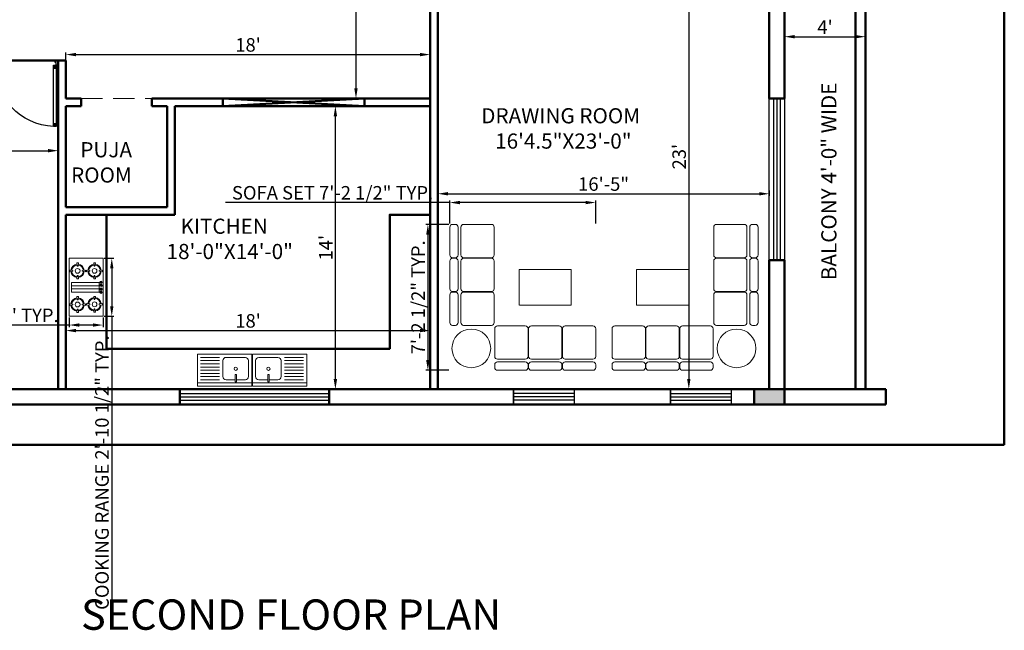
# Model space of a CAD drawing. Units: millimetres. Extents: x 1706 to 5913, y 156 to 1716.
# Tile 3 of 26: x 2060 to 2643, y 211 to 573. Entities that reach past the tile are written whole.
import ezdxf

# ---------------------------------------------------------------- set-up
doc = ezdxf.new("R2010")
doc.units = ezdxf.units.MM
doc.linetypes.add('DASHED', pattern=[19.05, 12.7, -6.35])
for name, color, linetype, lineweight in [('A-ANNO-DIMS', 2, 'Continuous', 18), ('A-ANNO-TEXT', 7, 'Continuous', 18), ('A-AREA-IDEN', 3, 'Continuous', 18), ('A-COLS', 20, 'Continuous', 50), ('A-DOOR', 4, 'Continuous', 25), ('A-FLOR-OVHD', 9, 'DASHED', 18), ('A-FURN', 8, 'Continuous', 18), ('A-GLAZ', 150, 'Continuous', 25), ('A-WALL', 7, 'Continuous', 50)]:
    doc.layers.add(name, color=color, linetype=linetype, lineweight=lineweight)
doc.styles.get("Standard").update_dxf_attribs({"font": 'arial.ttf'})
doc.dimstyles.new('ISO-25', dxfattribs={"dimtxt": 8, "dimasz": 6, "dimexe": 1.25, "dimexo": 0.625, "dimtad": 1, "dimdec": 0, "dimlunit": 3, "dimtxsty": 'Standard', "dimcen": 2.5, "dimadec": 0, "dimazin": 0, "dimtfac": 1, "dimtdec": 0, "dimtmove": 0, "dimatfit": 3, "dimfxl": 1, "dimarcsym": 0})

# ---------------------------------------------------------------- blocks, each defined once
blk = doc.blocks.new('Puerta 01')
for p, q in [((-0.775, -0.026), (-0.737, -0.058)), ((-0.775, -0.058), (-0.737, -0.026)), ((-0.737, -0.058), (-0.737, -0.026)), ((-0.028, -0.058), (-0.066, -0.026)), ((-0.028, -0.026), (-0.066, -0.058)), ((-0.066, -0.058), (-0.066, -0.026))]:
    blk.add_line(p, q)
for points in [[(-0.028, 0), (-0.028, -0.026), (0.004, -0.026), (0.004, -0.036), (0.028, -0.036), (0.028, 0)], [(-0.028, -0.026), (-0.775, -0.026), (-0.775, -0.058), (-0.028, -0.058)], [(0.004, -0.774), (0.004, -0.764), (0.028, -0.764), (0.028, -0.8), (-0.028, -0.8), (-0.028, -0.774)]]:
    blk.add_lwpolyline(points, close=True)
blk.add_arc((-0.028, -0.026), 0.747, 182.4545, 270)
blk = doc.blocks.new('A$C57CF26DA')
for p, q in [((0, 0), (0, 420)), ((720, 420), (0, 420)), ((167, 413), (147, 413)), ((147, 413), (152, 373)), ((152, 373), (162, 373)), ((162, 373), (167, 413)), ((300, 391), (300, 49)), ((300, 391), (420, 391)), ((340, 391), (340, 49)), ((380, 391), (380, 49)), ((420, 391), (420, 49)), ((584, 413), (564, 413)), ((564, 413), (569, 373)), ((569, 373), (579, 373)), ((579, 373), (584, 413)), ((720, 0), (720, 420)), ((99, 320), (59, 325)), ((59, 325), (59, 305)), ((59, 305), (99, 310)), ((99, 310), (99, 320)), ((152, 257), (147, 217)), ((162, 257), (152, 257)), ((167, 217), (162, 257)), ((255, 325), (215, 320)), ((215, 320), (215, 310)), ((215, 310), (255, 305)), ((255, 305), (255, 325)), ((516, 320), (476, 325)), ((476, 325), (476, 305)), ((476, 305), (516, 310)), ((516, 310), (516, 320)), ((569, 257), (564, 217)), ((579, 257), (569, 257)), ((584, 217), (579, 257)), ((672, 325), (632, 320)), ((632, 320), (632, 310)), ((632, 310), (672, 305)), ((672, 305), (672, 325)), ((147, 217), (167, 217)), ((167, 203), (147, 203)), ((147, 203), (152, 163)), ((152, 163), (162, 163)), ((162, 163), (167, 203)), ((581, 203), (561, 203)), ((561, 203), (566, 163)), ((564, 217), (584, 217)), ((566, 163), (576, 163)), ((576, 163), (581, 203)), ((99, 110), (59, 115)), ((59, 115), (59, 95)), ((59, 95), (99, 100)), ((99, 100), (99, 110)), ((152, 47), (147, 7)), ((147, 7), (167, 7)), ((162, 47), (152, 47)), ((167, 7), (162, 47)), ((255, 115), (215, 110)), ((215, 110), (215, 100)), ((215, 100), (255, 95)), ((255, 95), (255, 115)), ((302, 39), (295, 39)), ((295, 39), (295, 11)), ((295, 11), (302, 11)), ((420, 49), (300, 49)), ((302, 11), (302, 39)), ((341, 39), (334, 39)), ((334, 39), (334, 11)), ((334, 11), (341, 11)), ((341, 11), (341, 39)), ((380, 11), (380, 39)), ((380, 39), (386, 39)), ((386, 11), (380, 11)), ((386, 39), (386, 11)), ((419, 11), (419, 39)), ((419, 39), (426, 39)), ((426, 11), (419, 11)), ((426, 39), (426, 11)), ((513, 110), (473, 115)), ((473, 115), (473, 95)), ((473, 95), (513, 100)), ((513, 100), (513, 110)), ((566, 47), (561, 7)), ((561, 7), (581, 7)), ((576, 47), (566, 47)), ((581, 7), (576, 47)), ((669, 115), (629, 110)), ((629, 110), (629, 100)), ((629, 100), (669, 95)), ((669, 95), (669, 115)), ((720, 0), (0, 0))]:
    blk.add_line(p, q)
for centre in [(157, 315), (574, 315), (157, 105), (571, 105)]:
    blk.add_circle(centre, 30)
for centre, radius, start, end in [((157, 315), 83, 95.5849, 174.4151), ((157, 315), 73, 95.3738, 174.6262), ((157, 315), 73, 5.3738, 84.6262), ((157, 315), 83, 5.5849, 84.4151), ((574, 315), 83, 95.5849, 174.4151), ((574, 315), 73, 95.3738, 174.6262), ((574, 315), 73, 5.3738, 84.6262), ((574, 315), 83, 5.5849, 84.4151), ((157, 315), 83, 185.5849, 264.4151), ((157, 315), 73, 185.3738, 264.6262), ((157, 315), 73, 275.3738, 354.6262), ((157, 315), 83, 275.5849, 354.4151), ((574, 315), 83, 185.5849, 264.4151), ((574, 315), 73, 185.3738, 264.6262), ((574, 315), 73, 275.3738, 354.6262), ((574, 315), 83, 275.5849, 354.4151), ((157, 105), 83, 95.5849, 174.4151), ((157, 105), 73, 95.3738, 174.6262), ((157, 105), 73, 5.3738, 84.6262), ((157, 105), 83, 5.5849, 84.4151), ((571, 105), 83, 95.5849, 174.4151), ((571, 105), 73, 95.3738, 174.6262), ((571, 105), 73, 5.3738, 84.6262), ((571, 105), 83, 5.5849, 84.4151), ((157, 105), 83, 185.5849, 264.4151), ((157, 105), 73, 185.3738, 264.6262), ((157, 105), 73, 275.3738, 354.6262), ((157, 105), 83, 275.5849, 354.4151), ((298, 25), 13.7, 104.4775, 255.5225), ((298, 25), 13.7, 284.4775, 75.5225), ((337, 25), 13.7, 104.4775, 255.5225), ((337, 25), 13.7, 284.4775, 75.5225), ((383, 25), 13.7, 104.4775, 255.5225), ((383, 25), 13.7, 284.4775, 75.5225), ((422, 25), 13.7, 104.4775, 255.5225), ((422, 25), 13.7, 284.4775, 75.5225), ((571, 105), 83, 185.5849, 264.4151), ((571, 105), 73, 185.3738, 264.6262), ((571, 105), 73, 275.3738, 354.6262), ((571, 105), 83, 275.5849, 354.4151)]:
    blk.add_arc(centre, radius, start, end)
blk = doc.blocks.new('A$C3404121D')
for p, q in [((0, 0), (0, 500)), ((0, 500), (850, 500)), ((850, 500), (850, 0)), ((0, 450), (850, 450)), ((50, 100), (50, 350)), ((100, 400), (240, 400)), ((240, 431), (240, 425)), ((260, 431), (240, 431)), ((240, 425), (240, 315)), ((240, 315), (260, 315)), ((260, 431), (260, 315)), ((260, 400), (400, 400)), ((450, 100), (450, 350)), ((502, 400), (801, 400)), ((502, 350), (801, 350)), ((502, 300), (801, 300)), ((502, 250), (801, 250)), ((502, 200), (801, 200)), ((850, 0), (0, 0)), ((400, 50), (100, 50)), ((502, 150), (801, 150)), ((502, 100), (801, 100)), ((801, 50), (502, 50))]:
    blk.add_line(p, q)
blk.add_circle((250, 228), 25)
for centre, start, end in [((100, 350), 90, 180), ((400, 350), 0, 90), ((100, 100), 180, 270), ((400, 100), 270, 0)]:
    blk.add_arc(centre, 50, start, end)
blk = doc.blocks.new('A$C753D6792')
at = {"linetype": 'ByBlock'}
for p, q in [((0, 2530), (0, 2580)), ((50, 2630), (550, 2630)), ((600, 2580), (600, 2530)), ((610, 2530), (610, 2580)), ((660, 2630), (1160, 2630)), ((1210, 2580), (1210, 2530)), ((1220, 2530), (1220, 2580)), ((1270, 2630), (1770, 2630)), ((1820, 2580), (1820, 2530)), ((0, 1880), (0, 2380)), ((550, 2480), (50, 2480)), ((550, 2430), (50, 2430)), ((600, 2380), (600, 1880)), ((610, 1880), (610, 2380)), ((1160, 2480), (660, 2480)), ((1160, 2430), (660, 2430)), ((1210, 2380), (1210, 1880)), ((1220, 1880), (1220, 2380)), ((1770, 2480), (1270, 2480)), ((1770, 2430), (1270, 2430)), ((1820, 1880), (1820, 2380)), ((50, 1830), (427, 1830)), ((387, 1830), (550, 1830)), ((660, 1830), (1037, 1830)), ((997, 1830), (1160, 1830)), ((1270, 1830), (1647, 1830)), ((1607, 1830), (1770, 1830)), ((1880, 1820), (2380, 1820)), ((2530, 1820), (2580, 1820)), ((1830, 1770), (1830, 1393)), ((2430, 1270), (2430, 1770)), ((2480, 1270), (2480, 1770)), ((2630, 1770), (2630, 1270)), ((442, 815), (442, 1455)), ((442, 1455), (1372, 1455)), ((1382, 1455), (1382, 815)), ((1830, 1433), (1830, 1270)), ((1830, 1160), (1830, 783)), ((2380, 1220), (1880, 1220)), ((1880, 1210), (2380, 1210)), ((2430, 660), (2430, 1160)), ((2480, 660), (2480, 1160)), ((2580, 1220), (2530, 1220)), ((2530, 1210), (2580, 1210)), ((2630, 1160), (2630, 660)), ((1382, 815), (442, 815)), ((1830, 823), (1830, 660)), ((1830, 550), (1830, 173)), ((2380, 610), (1880, 610)), ((1880, 600), (2380, 600)), ((2430, 50), (2430, 550)), ((2480, 50), (2480, 550)), ((2580, 610), (2530, 610)), ((2530, 600), (2580, 600)), ((2630, 550), (2630, 50)), ((1830, 213), (1830, 50)), ((2380, 0), (1880, 0)), ((2580, 0), (2530, 0))]:
    blk.add_line(p, q, dxfattribs=at)
blk.add_circle((2242, 2235), 349, dxfattribs=at)
for centre, start, end in [((50, 2580), 90, 180), ((50, 2530), 180, 270), ((550, 2580), 0, 90), ((550, 2580), 0, 90), ((550, 2530), 270, 0), ((550, 2530), 270, 0), ((660, 2580), 90, 180), ((660, 2530), 180, 270), ((1160, 2580), 0, 90), ((1160, 2580), 0, 90), ((1160, 2530), 270, 0), ((1160, 2530), 270, 0), ((1270, 2580), 90, 180), ((1270, 2530), 180, 270), ((1770, 2580), 0, 90), ((1770, 2580), 0, 90), ((1770, 2530), 270, 0), ((1770, 2530), 270, 0), ((50, 2380), 90, 180), ((550, 2380), 0, 90), ((550, 2380), 0, 90), ((660, 2380), 90, 180), ((1160, 2380), 0, 90), ((1160, 2380), 0, 90), ((1270, 2380), 90, 180), ((1770, 2380), 0, 90), ((1770, 2380), 0, 90), ((50, 1880), 180, 270), ((550, 1880), 270, 0), ((660, 1880), 180, 270), ((1160, 1880), 270, 0), ((1270, 1880), 180, 270), ((1770, 1880), 270, 0), ((1880, 1770), 90, 180), ((2380, 1770), 0, 90), ((2530, 1770), 90, 180), ((2580, 1770), 0, 90), ((1880, 1270), 180, 270), ((2380, 1270), 270, 0), ((2380, 1270), 270, 0), ((2530, 1270), 180, 270), ((2530, 1270), 180, 270), ((2580, 1270), 270, 0), ((2580, 1270), 270, 0), ((1880, 1160), 90, 180), ((2380, 1160), 0, 90), ((2530, 1160), 90, 180), ((2580, 1160), 0, 90), ((1880, 660), 180, 270), ((1880, 550), 90, 180), ((2380, 660), 270, 0), ((2380, 660), 270, 0), ((2380, 550), 0, 90), ((2530, 660), 180, 270), ((2530, 660), 180, 270), ((2530, 550), 90, 180), ((2580, 660), 270, 0), ((2580, 660), 270, 0), ((2580, 550), 0, 90), ((1880, 50), 180, 270), ((2380, 50), 270, 0), ((2380, 50), 270, 0), ((2530, 50), 180, 270), ((2530, 50), 180, 270), ((2580, 50), 270, 0), ((2580, 50), 270, 0)]:
    blk.add_arc(centre, 50, start, end, dxfattribs=at)
blk = doc.blocks.new('*D119')
at = {"layer": 'A-ANNO-DIMS', "color": 0, "lineweight": -2, "transparency": 16777216}
for p, q in [((1801.94, 495.25), (1801.94, 496.83)), ((2082.44, 495.25), (2082.44, 496.83)), ((1807.94, 495.58), (2076.44, 495.58))]:
    blk.add_line(p, q, dxfattribs=at)
at = {"layer": 'A-ANNO-DIMS', "color": 0, "transparency": 16777216}
for points in [[(1807.94, 496.58), (1807.94, 494.58), (1801.94, 495.58)], [(2076.44, 496.58), (2076.44, 494.58), (2082.44, 495.58)]]:
    blk.add_solid(points, dxfattribs=at)
at = {"layer": 'Defpoints', "color": 0, "transparency": 16777216}
for p in [(1801.94, 494.63), (2082.44, 495.58), (2082.44, 494.63)]:
    blk.add_point(p, dxfattribs=at)
at = {"layer": 'A-ANNO-DIMS', "color": 0, "transparency": 16777216, "insert": (1942.19, 500.29), "char_height": 8, "attachment_point": 5}
blk.add_mtext('23\'-5"', dxfattribs=at)
blk = doc.blocks.new('*D136')
at = {"layer": 'A-ANNO-DIMS', "color": 0, "lineweight": -2, "transparency": 16777216}
for p, q in [((2256.32, 684.04), (2260.17, 684.04)), ((2258.92, 678.04), (2258.92, 532.54)), ((2256.32, 526.54), (2260.17, 526.54))]:
    blk.add_line(p, q, dxfattribs=at)
at = {"layer": 'A-ANNO-DIMS', "color": 0, "transparency": 16777216}
for points in [[(2257.92, 678.04), (2259.92, 678.04), (2258.92, 684.04)], [(2257.92, 532.54), (2259.92, 532.54), (2258.92, 526.54)]]:
    blk.add_solid(points, dxfattribs=at)
at = {"layer": 'Defpoints', "color": 0, "transparency": 16777216}
for p in [(2255.69, 684.04), (2255.69, 526.54), (2258.92, 526.54)]:
    blk.add_point(p, dxfattribs=at)
at = {"layer": 'A-ANNO-DIMS', "color": 0, "transparency": 16777216, "insert": (2254.2, 605.29), "char_height": 8, "attachment_point": 5, "rotation": 90}
blk.add_mtext('13\'-2"', dxfattribs=at)
blk = doc.blocks.new('*D137')
at = {"layer": 'A-ANNO-DIMS', "color": 0, "lineweight": -2, "transparency": 16777216}
for p, q in [((2086.94, 540.29), (2086.94, 553.85)), ((2092.94, 552.6), (2296.94, 552.6)), ((2302.94, 540.29), (2302.94, 553.85))]:
    blk.add_line(p, q, dxfattribs=at)
at = {"layer": 'A-ANNO-DIMS', "color": 0, "transparency": 16777216}
for points in [[(2092.94, 553.6), (2092.94, 551.6), (2086.94, 552.6)], [(2296.94, 553.6), (2296.94, 551.6), (2302.94, 552.6)]]:
    blk.add_solid(points, dxfattribs=at)
at = {"layer": 'Defpoints', "color": 0, "transparency": 16777216}
for p in [(2302.94, 552.6), (2086.94, 539.66), (2302.94, 539.66)]:
    blk.add_point(p, dxfattribs=at)
at = {"layer": 'A-ANNO-DIMS', "color": 0, "transparency": 16777216, "insert": (2194.94, 557.31), "char_height": 8, "attachment_point": 5}
blk.add_mtext("18'", dxfattribs=at)
blk = doc.blocks.new('*D138')
at = {"layer": 'A-ANNO-DIMS', "color": 0, "lineweight": -2, "transparency": 16777216}
for p, q in [((2247.7, 522.04), (2245.46, 522.04)), ((2246.71, 360.04), (2246.71, 516.04)), ((2247.7, 354.04), (2245.46, 354.04))]:
    blk.add_line(p, q, dxfattribs=at)
at = {"layer": 'A-ANNO-DIMS', "color": 0, "transparency": 16777216}
for points in [[(2245.71, 516.04), (2247.71, 516.04), (2246.71, 522.04)], [(2245.71, 360.04), (2247.71, 360.04), (2246.71, 354.04)]]:
    blk.add_solid(points, dxfattribs=at)
at = {"layer": 'Defpoints', "color": 0, "transparency": 16777216}
for p in [(2246.71, 522.04), (2248.33, 522.04), (2248.33, 354.04)]:
    blk.add_point(p, dxfattribs=at)
at = {"layer": 'A-ANNO-DIMS', "color": 0, "transparency": 16777216, "insert": (2242.07, 438.04), "char_height": 8, "attachment_point": 5, "rotation": 90}
blk.add_mtext("14'", dxfattribs=at)
blk = doc.blocks.new('*D139')
at = {"layer": 'A-ANNO-DIMS', "color": 0, "lineweight": -2, "transparency": 16777216}
for p, q in [((2086.94, 381.5), (2086.94, 390.09)), ((2092.94, 388.84), (2296.94, 388.84)), ((2302.94, 381.5), (2302.94, 390.09))]:
    blk.add_line(p, q, dxfattribs=at)
at = {"layer": 'A-ANNO-DIMS', "color": 0, "transparency": 16777216}
for points in [[(2092.94, 389.84), (2092.94, 387.84), (2086.94, 388.84)], [(2296.94, 389.84), (2296.94, 387.84), (2302.94, 388.84)]]:
    blk.add_solid(points, dxfattribs=at)
at = {"layer": 'Defpoints', "color": 0, "transparency": 16777216}
for p in [(2302.94, 388.84), (2086.94, 380.87), (2302.94, 380.87)]:
    blk.add_point(p, dxfattribs=at)
at = {"layer": 'A-ANNO-DIMS', "color": 0, "transparency": 16777216, "insert": (2194.94, 393.55), "char_height": 8, "attachment_point": 5}
blk.add_mtext("18'", dxfattribs=at)
blk = doc.blocks.new('*D140')
at = {"layer": 'A-ANNO-DIMS', "color": 0, "lineweight": -2, "transparency": 16777216}
for p, q in [((2452.75, 630.04), (2457.47, 630.04)), ((2456.22, 624.04), (2456.22, 360.04)), ((2452.75, 354.04), (2457.47, 354.04))]:
    blk.add_line(p, q, dxfattribs=at)
at = {"layer": 'A-ANNO-DIMS', "color": 0, "transparency": 16777216}
for points in [[(2455.22, 624.04), (2457.22, 624.04), (2456.22, 630.04)], [(2455.22, 360.04), (2457.22, 360.04), (2456.22, 354.04)]]:
    blk.add_solid(points, dxfattribs=at)
at = {"layer": 'Defpoints', "color": 0, "transparency": 16777216}
for p in [(2452.12, 630.04), (2452.12, 354.04), (2456.22, 354.04)]:
    blk.add_point(p, dxfattribs=at)
at = {"layer": 'A-ANNO-DIMS', "color": 0, "transparency": 16777216, "insert": (2451.51, 492.04), "char_height": 8, "attachment_point": 5, "rotation": 90}
blk.add_mtext("23'", dxfattribs=at)
blk = doc.blocks.new('*D141')
at = {"layer": 'A-ANNO-DIMS', "color": 0, "lineweight": -2, "transparency": 16777216}
for p, q in [((2307.44, 471.91), (2307.44, 468.77)), ((2313.44, 470.02), (2497.94, 470.02)), ((2503.94, 471.91), (2503.94, 468.77))]:
    blk.add_line(p, q, dxfattribs=at)
at = {"layer": 'A-ANNO-DIMS', "color": 0, "transparency": 16777216}
for points in [[(2313.44, 471.02), (2313.44, 469.02), (2307.44, 470.02)], [(2497.94, 471.02), (2497.94, 469.02), (2503.94, 470.02)]]:
    blk.add_solid(points, dxfattribs=at)
at = {"layer": 'Defpoints', "color": 0, "transparency": 16777216}
for p in [(2307.44, 472.54), (2503.94, 472.54), (2503.94, 470.02)]:
    blk.add_point(p, dxfattribs=at)
at = {"layer": 'A-ANNO-DIMS', "color": 0, "transparency": 16777216, "insert": (2405.69, 474.73), "char_height": 8, "attachment_point": 5}
blk.add_mtext('16\'-5"', dxfattribs=at)
blk = doc.blocks.new('*D143')
at = {"layer": 'A-ANNO-DIMS', "color": 0, "lineweight": -2, "transparency": 16777216}
for p, q in [((2512.94, 564.2), (2512.94, 561.96)), ((2518.94, 563.21), (2554.94, 563.21)), ((2560.94, 564.2), (2560.94, 561.96))]:
    blk.add_line(p, q, dxfattribs=at)
at = {"layer": 'A-ANNO-DIMS', "color": 0, "transparency": 16777216}
for points in [[(2518.94, 564.21), (2518.94, 562.21), (2512.94, 563.21)], [(2554.94, 564.21), (2554.94, 562.21), (2560.94, 563.21)]]:
    blk.add_solid(points, dxfattribs=at)
at = {"layer": 'Defpoints', "color": 0, "transparency": 16777216}
for p in [(2512.94, 564.83), (2560.94, 564.83), (2560.94, 563.21)]:
    blk.add_point(p, dxfattribs=at)
at = {"layer": 'A-ANNO-DIMS', "color": 0, "transparency": 16777216, "insert": (2536.94, 567.84), "char_height": 8, "attachment_point": 5}
blk.add_mtext("4'", dxfattribs=at)
blk = doc.blocks.new('*D225')
at = {"layer": 'A-ANNO-DIMS', "color": 0, "lineweight": -2, "transparency": 16777216}
for p, q in [((2314.52, 464.8), (2181.53, 464.8)), ((2314.52, 452.44), (2314.52, 466.05)), ((2395.06, 464.8), (2320.52, 464.8)), ((2401.06, 452.44), (2401.06, 466.05))]:
    blk.add_line(p, q, dxfattribs=at)
at = {"layer": 'A-ANNO-DIMS', "color": 0, "transparency": 16777216}
for points in [[(2320.52, 465.8), (2320.52, 463.8), (2314.52, 464.8)], [(2395.06, 465.8), (2395.06, 463.8), (2401.06, 464.8)]]:
    blk.add_solid(points, dxfattribs=at)
at = {"layer": 'Defpoints', "color": 0, "transparency": 16777216}
for p in [(2314.52, 464.8), (2314.52, 451.82), (2401.06, 451.82)]:
    blk.add_point(p, dxfattribs=at)
at = {"layer": 'A-ANNO-DIMS', "color": 0, "transparency": 16777216, "insert": (2245.03, 469.56), "char_height": 8, "attachment_point": 5}
blk.add_mtext('SOFA SET 7\'-2 1/2" TYP.', dxfattribs=at)
blk = doc.blocks.new('*D226')
at = {"layer": 'A-ANNO-DIMS', "color": 0, "lineweight": -2, "transparency": 16777216}
for p, q in [((2313.9, 451.82), (2300.29, 451.82)), ((2301.54, 445.82), (2301.54, 371.28)), ((2313.9, 365.28), (2300.29, 365.28))]:
    blk.add_line(p, q, dxfattribs=at)
at = {"layer": 'A-ANNO-DIMS', "color": 0, "transparency": 16777216}
for points in [[(2300.54, 445.82), (2302.54, 445.82), (2301.54, 451.82)], [(2300.54, 371.28), (2302.54, 371.28), (2301.54, 365.28)]]:
    blk.add_solid(points, dxfattribs=at)
at = {"layer": 'Defpoints', "color": 0, "transparency": 16777216}
for p in [(2314.52, 451.82), (2301.54, 365.28), (2314.52, 365.28)]:
    blk.add_point(p, dxfattribs=at)
at = {"layer": 'A-ANNO-DIMS', "color": 0, "transparency": 16777216, "insert": (2296.78, 408.55), "char_height": 8, "attachment_point": 5, "rotation": 90}
blk.add_mtext('7\'-2 1/2" TYP.', dxfattribs=at)
blk = doc.blocks.new('*D229')
at = {"layer": 'A-ANNO-DIMS', "color": 0, "lineweight": -2, "transparency": 16777216}
for p, q in [((2109.61, 431.76), (2115.4, 431.76)), ((2114.15, 425.76), (2114.15, 403.29)), ((2109.61, 397.29), (2115.4, 397.29)), ((2114.15, 397.29), (2114.15, 217.78))]:
    blk.add_line(p, q, dxfattribs=at)
at = {"layer": 'A-ANNO-DIMS', "color": 0, "transparency": 16777216}
for points in [[(2113.15, 425.76), (2115.15, 425.76), (2114.15, 431.76)], [(2113.15, 403.29), (2115.15, 403.29), (2114.15, 397.29)]]:
    blk.add_solid(points, dxfattribs=at)
at = {"layer": 'Defpoints', "color": 0, "transparency": 16777216}
for p in [(2108.98, 431.76), (2108.98, 397.29), (2114.15, 397.29)]:
    blk.add_point(p, dxfattribs=at)
at = {"layer": 'A-ANNO-DIMS', "color": 0, "transparency": 16777216, "insert": (2109.39, 304.54), "char_height": 8, "attachment_point": 5, "rotation": 90}
blk.add_mtext('COOKING RANGE 2\'-10 1/2" TYP.', dxfattribs=at)
blk = doc.blocks.new('*D230')
at = {"layer": 'A-ANNO-DIMS', "color": 0, "lineweight": -2, "transparency": 16777216}
for p, q in [((2088.87, 392.12), (2033.61, 392.12)), ((2088.87, 396.67), (2088.87, 390.87)), ((2102.98, 392.12), (2094.87, 392.12)), ((2108.98, 396.67), (2108.98, 390.87))]:
    blk.add_line(p, q, dxfattribs=at)
at = {"layer": 'A-ANNO-DIMS', "color": 0, "transparency": 16777216}
for points in [[(2094.87, 393.12), (2094.87, 391.12), (2088.87, 392.12)], [(2102.98, 393.12), (2102.98, 391.12), (2108.98, 392.12)]]:
    blk.add_solid(points, dxfattribs=at)
at = {"layer": 'Defpoints', "color": 0, "transparency": 16777216}
for p in [(2088.87, 397.29), (2108.98, 397.29), (2088.87, 392.12)]:
    blk.add_point(p, dxfattribs=at)
at = {"layer": 'A-ANNO-DIMS', "color": 0, "transparency": 16777216, "insert": (2058.24, 396.83), "char_height": 8, "attachment_point": 5}
blk.add_mtext('1\'-8" TYP.', dxfattribs=at)

msp = doc.modelspace()

# ---------------------------------------------------------------- hatches: boundary and pattern name
at = {"layer": 'A-COLS'}
h = msp.add_hatch(color=256, dxfattribs=at)
h.dxf.hatch_style = 1
h.paths.add_polyline_path([(2512.94, 354.04), (2494.94, 354.04), (2494.94, 345.04), (2512.94, 345.04)])

# ---------------------------------------------------------------- linework, layer by layer
msp.add_lwpolyline([(2513.16, 354.04), (2494.94, 354.04), (2494.94, 345.04), (2512.94, 345.04), (2512.94, 354.04)], dxfattribs=at)
at = {"layer": 'A-FLOR-OVHD'}
msp.add_line((2095.94, 526.54), (2137.94, 526.54), dxfattribs=at)
at = {"layer": 'A-GLAZ'}
for p, q in [((2506.44, 526.54), (2506.44, 430.54)), ((2508.44, 526.54), (2508.44, 430.54)), ((2510.44, 526.54), (2510.44, 430.54)), ((2154.44, 351.54), (2242.94, 351.54)), ((2352.3, 354.04), (2352.3, 345.04)), ((2388.3, 351.54), (2352.3, 351.54)), ((2388.3, 354.04), (2388.3, 345.04)), ((2445.3, 354.04), (2445.3, 345.04)), ((2445.3, 351.54), (2481.3, 351.54)), ((2481.3, 354.04), (2481.3, 345.04)), ((2154.44, 349.54), (2242.94, 349.54)), ((2154.44, 347.54), (2242.94, 347.54)), ((2388.3, 349.54), (2352.3, 349.54)), ((2388.3, 347.54), (2352.3, 347.54)), ((2445.3, 349.54), (2481.3, 349.54)), ((2445.3, 347.54), (2481.3, 347.54))]:
    msp.add_line(p, q, dxfattribs=at)
for points in [[(2503.94, 526.54), (2512.94, 526.54), (2512.94, 430.54), (2503.94, 430.54)], [(2154.44, 354.04), (2242.94, 354.04), (2242.94, 345.04), (2154.44, 345.04)], [(2352.3, 354.04), (2388.3, 354.04), (2388.3, 345.04), (2352.3, 345.04)], [(2445.3, 354.04), (2481.3, 354.04), (2481.3, 345.04), (2445.3, 345.04)]]:
    msp.add_lwpolyline(points, close=True, dxfattribs=at)
at = {"layer": 'A-WALL'}
for p, q in [((2643.23, 844.54), (2643.23, 321.04)), ((2554.94, 622.54), (2554.94, 354.04)), ((2560.94, 622.54), (2560.94, 354.04)), ((2302.94, 591.04), (2302.94, 354.04)), ((2307.44, 591.04), (2307.44, 354.04)), ((2503.94, 583.54), (2503.94, 526.54)), ((2512.94, 583.54), (2512.94, 526.54)), ((2043.44, 549.04), (2082.44, 549.04)), ((2082.44, 549.04), (2082.44, 354.04)), ((2082.44, 549.04), (2086.94, 549.04)), ((2086.94, 549.04), (2086.94, 526.54)), ((2086.94, 526.54), (2095.94, 526.54)), ((2095.94, 526.54), (2095.94, 522.04)), ((2137.94, 526.54), (2137.94, 522.04)), ((2137.94, 526.54), (2179.94, 526.54)), ((2179.94, 526.54), (2179.94, 522.04)), ((2263.94, 526.54), (2179.94, 522.04)), ((2179.94, 526.54), (2263.94, 522.04)), ((2263.94, 526.54), (2263.94, 522.04)), ((2263.94, 526.54), (2302.94, 526.54)), ((2512.94, 526.54), (2503.94, 526.54)), ((2086.94, 522.04), (2086.94, 462.04)), ((2086.94, 522.04), (2095.94, 522.04)), ((2137.94, 522.04), (2146.94, 522.04)), ((2146.94, 522.04), (2146.94, 462.04)), ((2151.44, 522.04), (2151.44, 457.54)), ((2151.44, 522.04), (2179.94, 522.04)), ((2263.94, 522.04), (2302.94, 522.04)), ((2086.94, 462.04), (2146.94, 462.04)), ((2086.94, 457.54), (2086.94, 354.04)), ((2086.94, 457.54), (2151.44, 457.54)), ((2503.94, 430.54), (2503.94, 354.04)), ((2512.94, 430.54), (2503.94, 430.54)), ((2512.94, 430.54), (2512.94, 354.04)), ((1777.94, 354.04), (2572.94, 354.04)), ((2154.44, 354.04), (2154.44, 345.04)), ((2242.94, 354.04), (2242.94, 345.04)), ((2512.94, 354.04), (2512.94, 345.04)), ((2512.94, 345.04), (2512.94, 354.04)), ((2572.94, 354.04), (2572.94, 345.04)), ((1773.44, 345.04), (2572.94, 345.04)), ((1747.94, 321.04), (2643.23, 321.04))]:
    msp.add_line(p, q, dxfattribs=at)
msp.add_lwpolyline([(2179.94, 526.54), (2263.94, 526.54), (2263.94, 522.04), (2179.94, 522.04)], close=True, dxfattribs=at)
msp.add_lwpolyline([(2110.94, 457.54), (2110.94, 378.04), (2278.94, 378.04), (2278.94, 457.54), (2302.94, 457.54)], dxfattribs=at)

# ---------------------------------------------------------------- block references
at = {"layer": 'A-DOOR', "extrusion": (0, 0, -1), "xscale": 48.75000000000294, "yscale": 48.75000000000294, "zscale": -48.75000000000287, "rotation": 89.99999999879581}
msp.add_blockref('Puerta 01', (-2082.44, 547.67), dxfattribs=at)
at = {"layer": 'A-FURN'}
for name, p, xscale, yscale, zscale, rotation in [('A$C753D6792', (2401.06, 451.82), 0.0329035460231199, 0.0329035460231199, 0.0329035460231199, 180), ('A$C753D6792', (2410.74, 451.82), -0.0329035460231199, 0.0329035460231199, 0.0329035460231199, 180), ('A$C57CF26DA', (2108.98, 431.76), -0.0478777176975714, 0.0478777176975714, 0.0478777176975714, 90), ('A$C3404121D', (2197.12, 374.8), 0.0378984485580132, 0.0378984485580132, 0.0378984485580132, 180), ('A$C3404121D', (2197.53, 374.8), -0.0378984485580132, 0.0378984485580132, 0.0378984485580132, 180)]:
    msp.add_blockref(name, p, dxfattribs=dict(at, xscale=xscale, yscale=yscale, zscale=zscale, rotation=rotation))

# ---------------------------------------------------------------- texts
at = {"layer": 'A-ANNO-TEXT', "insert": (2095.94, 229.29), "char_height": 18, "attachment_point": 1}
msp.add_mtext_dynamic_manual_height_columns('SECOND FLOOR PLAN', width=352.5721, gutter_width=12.5, heights=[0], dxfattribs=at)
at = {"layer": 'A-AREA-IDEN', "insert": (2534.75, 407.73), "char_height": 9, "attachment_point": 1, "rotation": 90}
msp.add_mtext_dynamic_manual_height_columns('    BALCONY 4\'-0" WIDE', width=166.3136, gutter_width=12.5, heights=[0], dxfattribs=at)
at = {"layer": 'A-AREA-IDEN', "char_height": 9, "attachment_point": 1}
for s, width, insert in [('    DRAWING ROOM\\P       16\'4.5"X23\'-0"', 125.2434, (2322.15, 520.79)), ('  PUJA ROOM', 67.9131, (2090.03, 500.64)), ('    KITCHEN\\P 18\'-0"X14\'-0"', 99.443, (2143.9, 455.25))]:
    msp.add_mtext_dynamic_manual_height_columns(s, width=width, gutter_width=12.5, heights=[0], dxfattribs=dict(at, insert=insert))

# ---------------------------------------------------------------- dimensions: what is measured, and where the dimension line sits
at = {"layer": 'A-ANNO-DIMS'}
for base, p1, p2, picture, middle in [((2258.91677014, 526.5366453), (2255.6916327, 684.0366453), (2255.6916327, 526.5366453), '*D136', (2254.20445772, 605.2866453)), ((2456.22, 354.04), (2452.12, 630.04), (2452.12, 354.04), '*D140', (2451.51, 492.04)), ((2246.71, 522.04), (2248.33, 354.04), (2248.33, 522.04), '*D138', (2242.07, 438.04))]:
    dim = msp.add_linear_dim(base=base, p1=p1, p2=p2, angle=90, dimstyle='ISO-25', override={"dimclrd": 0, "dimclre": 0, "dimclrt": 0}, dxfattribs=at)
    dim.commit()
    dim.dimension.update_dxf_attribs({"geometry": picture, "text_midpoint": middle})
for base, p1, p2, picture, middle in [((2560.94, 563.21), (2512.94, 564.83), (2560.94, 564.83), '*D143', (2536.94, 567.84)), ((2302.94, 552.6), (2086.94, 539.66), (2302.94, 539.66), '*D137', (2194.94, 557.31)), ((2082.4416327, 495.58217097), (1801.9416327, 494.62714103), (2082.4416327, 494.62714103), '*D119', (1942.1916327, 500.29448338)), ((2503.9416327, 470.01909582), (2307.4416327, 472.5366453), (2503.9416327, 472.5366453), '*D141', (2405.6916327, 474.72867972)), ((2302.94, 388.84), (2086.94, 380.87), (2302.94, 380.87), '*D139', (2194.94, 393.55))]:
    dim = msp.add_linear_dim(base=base, p1=p1, p2=p2, dimstyle='ISO-25', override={"dimclrd": 0, "dimclre": 0, "dimclrt": 0}, dxfattribs=at)
    dim.commit()
    dim.dimension.update_dxf_attribs({"geometry": picture, "text_midpoint": middle})
for base, p1, p2, angle, text, picture, middle in [((2314.52, 464.8), (2401.06, 451.82), (2314.52, 451.82), 180, 'SOFA SET <> TYP.', '*D225', (2245.03, 469.56)), ((2301.54, 365.28), (2314.52, 451.82), (2314.52, 365.28), 270, '<> TYP.', '*D226', (2296.78, 408.55)), ((2114.15, 397.29), (2108.98, 431.76), (2108.98, 397.29), 270, 'COOKING RANGE <> TYP.', '*D229', (2109.39, 304.54)), ((2088.87, 392.12), (2108.98, 397.29), (2088.87, 397.29), 180, '<> TYP.', '*D230', (2058.24, 396.83))]:
    dim = msp.add_linear_dim(base=base, p1=p1, p2=p2, angle=angle, text=text, dimstyle='ISO-25', override={"dimdec": 1, "dimrnd": 0, "dimzin": 1, "dimlunit": 4, "dimfrac": 2}, dxfattribs=at)
    dim.commit()
    dim.dimension.update_dxf_attribs({"geometry": picture, "text_midpoint": middle})

doc.saveas('drawing.dxf')
